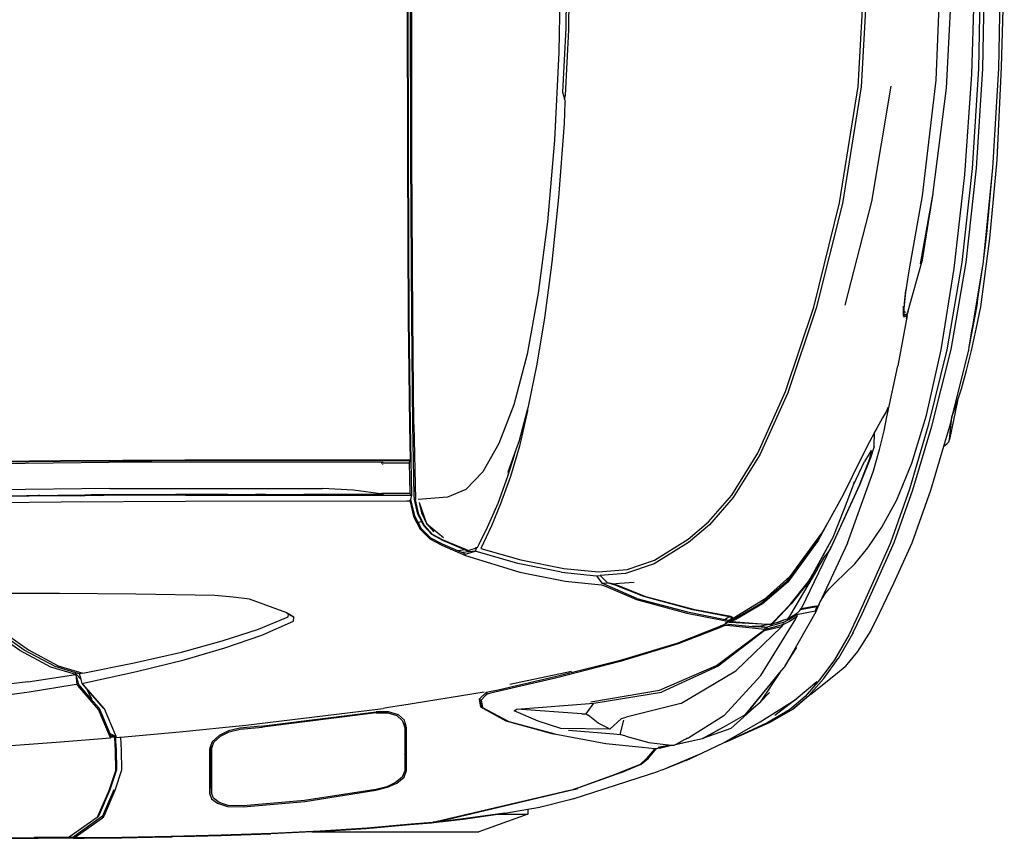
# Model space of a CAD drawing. Units: inches. Extents: x 22042254 to 25404563, y 17568978 to 17626777.
# Tile 16 of 45: x 22042342.6037 to 22042343.228, y 17568977.6632 to 17568978.1821. Entities that reach past the tile are written whole.
import ezdxf

# ---------------------------------------------------------------- set-up
doc = ezdxf.new("R2010")
doc.units = ezdxf.units.IN
doc.header["$MEASUREMENT"] = 0
doc.layers.add('A-SITE-VEHI', color=8, linetype='Continuous', lineweight=18)
doc.layers.add('Edges', color=250, linetype='Continuous')

# ---------------------------------------------------------------- blocks, each defined once
blk = doc.blocks.new('Nissan Qashqai pl')
at = {"layer": 'Edges'}
for p, q in [((10.6151, 12.8159), (10.6644, 12.8162)), ((10.6176, 12.8164), (10.6651, 12.8167)), ((10.6644, 12.8162), (10.7078, 12.8159)), ((10.6651, 12.8167), (10.666, 12.8167)), ((10.666, 12.8167), (10.677, 12.8167)), ((10.6729, 12.8157), (10.7082, 12.8156)), ((10.6809, 12.8167), (10.677, 12.8167)), ((10.7128, 12.8166), (10.6809, 12.8167)), ((10.7078, 12.8159), (10.7083, 12.8156)), ((10.7082, 12.8156), (10.7078, 12.8159)), ((10.7085, 12.8153), (10.7082, 12.8156)), ((10.7082, 12.8156), (10.7083, 12.8156)), ((10.7083, 12.8156), (10.7087, 12.8153)), ((10.7083, 12.8156), (10.7125, 12.8156)), ((10.7087, 12.8153), (10.7363, 12.7959)), ((10.7139, 12.8164), (10.7125, 12.8156)), ((10.7137, 12.8148), (10.7125, 12.8156)), ((10.7128, 12.8166), (10.7625, 12.8161)), ((10.7128, 12.8166), (10.724, 12.8166)), ((10.7139, 12.8164), (10.7148, 12.8157)), ((10.7628, 12.8158), (10.7139, 12.8164)), ((10.7148, 12.8157), (10.7429, 12.7956)), ((10.7685, 12.8161), (10.724, 12.8166)), ((10.7625, 12.8161), (10.7628, 12.8161)), ((10.7628, 12.8161), (10.8099, 12.8152)), ((10.8131, 12.8149), (10.7628, 12.8158)), ((10.7688, 12.8161), (10.7685, 12.8161)), ((10.8099, 12.8152), (10.7688, 12.8161)), ((10.8099, 12.8152), (10.8131, 12.8152)), ((10.8134, 12.8152), (10.8131, 12.8152)), ((10.8134, 12.8152), (10.8142, 12.8152)), ((10.8142, 12.8152), (10.8142, 12.8152)), ((10.8237, 12.8149), (10.8142, 12.8152)), ((10.7137, 12.8148), (10.7138, 12.8147)), ((10.7418, 12.7947), (10.7138, 12.8147)), ((10.8644, 12.8135), (10.8131, 12.8149)), ((10.8237, 12.8149), (10.864, 12.8138)), ((10.8596, 12.8138), (10.8589, 12.8138)), ((10.8642, 12.8136), (10.8596, 12.8138)), ((10.864, 12.8138), (10.8642, 12.8138)), ((10.8642, 12.8138), (10.9152, 12.812)), ((10.9158, 12.8118), (10.8644, 12.8135)), ((10.9577, 12.8101), (10.9152, 12.812)), ((10.9657, 12.8095), (10.9158, 12.8118)), ((10.9577, 12.8101), (10.9649, 12.8097)), ((10.9577, 12.8101), (11.1283, 12.8101)), ((10.9649, 12.8097), (11.0127, 12.8067)), ((11.0138, 12.8064), (10.9657, 12.8095)), ((11.0127, 12.8067), (11.0576, 12.8026)), ((11.059, 12.8023), (11.0138, 12.8064)), ((11.1783, 12.7921), (11.1283, 12.8101)), ((10.7363, 12.7959), (10.7376, 12.795)), ((10.7387, 12.794), (10.7376, 12.795)), ((10.7376, 12.795), (10.7378, 12.7946)), ((10.7432, 12.7954), (10.7426, 12.7954)), ((10.7429, 12.7956), (10.7432, 12.7954)), ((10.7441, 12.7954), (10.7432, 12.7954)), ((10.7432, 12.7954), (10.744, 12.7948)), ((11.0576, 12.8026), (11.0798, 12.8008)), ((11.0768, 12.8008), (11.059, 12.8023)), ((11.0811, 12.8004), (11.0768, 12.8008)), ((11.0798, 12.8008), (11.0872, 12.7999)), ((11.0827, 12.8001), (11.0811, 12.8004)), ((11.0827, 12.8001), (11.0813, 12.7998)), ((11.0836, 12.8002), (11.0827, 12.8001)), ((11.0856, 12.7994), (11.0827, 12.8001)), ((11.0872, 12.7999), (11.0836, 12.8002)), ((11.0836, 12.8002), (11.0882, 12.7992)), ((11.2196, 12.7681), (11.0856, 12.7994)), ((11.0883, 12.7998), (11.0872, 12.7999)), ((11.0882, 12.7992), (11.2222, 12.7676)), ((11.0883, 12.7998), (11.1123, 12.797)), ((11.1147, 12.7965), (11.0883, 12.7998)), ((11.1123, 12.797), (11.1475, 12.7921)), ((11.1547, 12.791), (11.1147, 12.7965)), ((10.7378, 12.7946), (10.7379, 12.7945)), ((10.7378, 12.7946), (10.7385, 12.7932)), ((10.7385, 12.7932), (10.7497, 12.7679)), ((10.7387, 12.794), (10.7396, 12.7922)), ((10.7396, 12.7922), (10.7507, 12.7669)), ((10.743, 12.7939), (10.7418, 12.7947)), ((10.7434, 12.793), (10.743, 12.7939)), ((10.7437, 12.7921), (10.7434, 12.793)), ((10.7438, 12.7921), (10.7437, 12.7921)), ((10.7438, 12.7921), (10.7549, 12.7666)), ((10.744, 12.7948), (10.7448, 12.793)), ((10.7448, 12.793), (10.7559, 12.7674)), ((11.1475, 12.7921), (11.1525, 12.7914)), ((11.1475, 12.7921), (11.1783, 12.7921)), ((11.1525, 12.7914), (11.1547, 12.791)), ((11.1547, 12.791), (11.1783, 12.787)), ((11.1783, 12.787), (11.1783, 12.7921)), ((11.1783, 12.787), (11.1906, 12.7849)), ((11.1906, 12.7849), (11.1909, 12.7849)), ((11.193, 12.7845), (11.1909, 12.7849)), ((10.8523, 12.7704), (10.8546, 12.7762)), ((10.8565, 12.7757), (10.8543, 12.7702)), ((10.8546, 12.7762), (10.8607, 12.7808)), ((10.8622, 12.7801), (10.8565, 12.7757)), ((10.8607, 12.7808), (10.8708, 12.7841)), ((10.8716, 12.7832), (10.8622, 12.7801)), ((10.8708, 12.7841), (10.8869, 12.7844)), ((10.887, 12.7835), (10.8716, 12.7832)), ((10.8869, 12.7844), (10.9499, 12.7789)), ((10.9498, 12.7781), (10.887, 12.7835)), ((11.0226, 12.7668), (10.9498, 12.7781)), ((10.9499, 12.7789), (11.0229, 12.7676)), ((11.2215, 12.7775), (11.193, 12.7845)), ((11.2247, 12.7764), (11.2215, 12.7775)), ((11.2247, 12.7764), (11.3124, 12.7479)), ((10.7497, 12.7679), (10.7565, 12.7473)), ((10.7507, 12.7669), (10.7575, 12.7462)), ((10.7559, 12.7674), (10.7626, 12.7467)), ((10.8523, 12.7255), (10.8523, 12.7704)), ((10.8543, 12.7702), (10.8538, 12.753)), ((10.8543, 12.7255), (10.8543, 12.7702)), ((11.0339, 12.7639), (11.0226, 12.7668)), ((11.0229, 12.7676), (11.0348, 12.7645)), ((11.2247, 12.767), (11.2163, 12.7689)), ((11.22, 12.768), (11.2196, 12.7681)), ((11.2247, 12.767), (11.22, 12.768)), ((11.2222, 12.7676), (11.2271, 12.7664)), ((11.2253, 12.7668), (11.2247, 12.767)), ((11.2304, 12.7649), (11.2253, 12.7668)), ((11.2253, 12.7668), (11.2271, 12.7664)), ((11.2271, 12.7664), (11.2296, 12.7658)), ((11.2271, 12.7664), (11.2277, 12.7662)), ((11.2277, 12.7662), (11.2296, 12.7658)), ((11.2732, 12.7496), (11.2277, 12.7662)), ((11.2704, 12.7504), (11.2304, 12.7649)), ((11.0429, 12.7597), (11.0339, 12.7639)), ((11.0348, 12.7645), (11.0444, 12.7601)), ((11.0497, 12.7542), (11.0429, 12.7597)), ((11.0444, 12.7601), (11.0516, 12.7542)), ((10.7565, 12.7473), (10.7563, 12.7273)), ((10.7575, 12.7462), (10.7572, 12.7263)), ((10.7626, 12.7467), (10.7623, 12.7269)), ((10.8528, 12.7503), (10.8535, 12.7521)), ((10.8528, 12.742), (10.8528, 12.7503)), ((10.8535, 12.7521), (10.8538, 12.753)), ((10.8538, 12.7521), (10.8535, 12.7521)), ((10.8538, 12.753), (10.8538, 12.7521)), ((10.8538, 12.7521), (10.8538, 12.7502)), ((10.8538, 12.7502), (10.8538, 12.742)), ((11.0523, 12.7475), (11.0497, 12.7542)), ((11.0516, 12.7542), (11.0543, 12.7473)), ((11.0528, 12.73), (11.0523, 12.7475)), ((11.0523, 12.7312), (11.0523, 12.7475)), ((11.0543, 12.7473), (11.0543, 12.7035)), ((11.2702, 12.7507), (11.2704, 12.7504)), ((11.2704, 12.7506), (11.2707, 12.7503)), ((11.2707, 12.7503), (11.2704, 12.7504)), ((11.2719, 12.7498), (11.2707, 12.7503)), ((11.2934, 12.741), (11.2719, 12.7498)), ((11.2732, 12.7496), (11.2946, 12.7409)), ((11.3161, 12.7467), (11.3124, 12.7479)), ((11.3161, 12.7467), (11.3376, 12.7381)), ((11.3192, 12.7454), (11.3566, 12.7294)), ((10.8528, 12.742), (10.8538, 12.742)), ((10.8528, 12.7419), (10.8528, 12.742)), ((10.8538, 12.7419), (10.8528, 12.7419)), ((10.8528, 12.7242), (10.8528, 12.7419)), ((10.8538, 12.742), (10.8538, 12.7419)), ((10.8538, 12.7214), (10.8538, 12.7419)), ((11.3, 12.735), (11.2934, 12.741)), ((11.2946, 12.7409), (11.3018, 12.7346)), ((11.3081, 12.7253), (11.3, 12.735)), ((11.3018, 12.7346), (11.3103, 12.7249)), ((11.3405, 12.7369), (11.3376, 12.7381)), ((11.3405, 12.7369), (11.3566, 12.7294)), ((10.7563, 12.7273), (10.7553, 12.7134)), ((10.7572, 12.7263), (10.7563, 12.7126)), ((10.7623, 12.7269), (10.7615, 12.7131)), ((10.8528, 12.7242), (10.8523, 12.7255)), ((10.8543, 12.7255), (10.8569, 12.7184)), ((11.0523, 12.7312), (11.0528, 12.73)), ((11.0523, 12.7287), (11.0523, 12.7312)), ((11.0528, 12.7274), (11.0523, 12.7287)), ((11.0523, 12.7037), (11.0523, 12.7287)), ((11.0528, 12.7274), (11.0528, 12.73)), ((11.0528, 12.73), (11.0538, 12.7273)), ((11.0528, 12.7274), (11.0528, 12.6985)), ((11.0538, 12.7273), (11.0538, 12.7018)), ((11.2956, 12.7234), (11.3085, 12.7247)), ((11.3086, 12.7247), (11.3081, 12.7253)), ((11.3081, 12.7253), (11.3087, 12.7247)), ((11.3085, 12.7247), (11.3086, 12.7247)), ((11.3086, 12.7247), (11.3087, 12.7247)), ((11.3087, 12.7247), (11.3103, 12.7249)), ((11.3103, 12.7249), (11.3103, 12.7249)), ((11.3103, 12.7249), (11.3106, 12.7249)), ((11.3106, 12.7249), (11.314, 12.7238)), ((11.3566, 12.7294), (11.3796, 12.7187)), ((10.6318, 12.7228), (10.6955, 12.7184)), ((10.6955, 12.7184), (10.7509, 12.714)), ((10.8538, 12.7214), (10.8528, 12.7242)), ((10.855, 12.7181), (10.8538, 12.7214)), ((10.8622, 12.7114), (10.855, 12.7181)), ((10.8569, 12.7184), (10.8637, 12.712)), ((11.2091, 12.7103), (11.2583, 12.7196)), ((11.2583, 12.7196), (11.2956, 12.7234)), ((11.2787, 12.7123), (11.3022, 12.7186)), ((11.3022, 12.7186), (11.3252, 12.7213)), ((11.317, 12.7227), (11.3119, 12.7236)), ((11.3132, 12.7243), (11.3256, 12.7215)), ((11.314, 12.7238), (11.317, 12.7227)), ((11.314, 12.7238), (11.3242, 12.7216)), ((11.3242, 12.7216), (11.317, 12.7227)), ((11.3198, 12.7211), (11.3252, 12.7213)), ((11.3242, 12.7216), (11.3256, 12.7215)), ((11.3252, 12.7213), (11.3283, 12.7214)), ((11.3256, 12.7215), (11.3283, 12.7214)), ((11.3283, 12.7214), (11.3297, 12.7206)), ((11.3297, 12.7206), (11.3446, 12.7173)), ((11.3297, 12.7206), (11.3302, 12.7203)), ((11.3302, 12.7203), (11.3446, 12.7173)), ((11.3302, 12.7203), (11.3394, 12.7152)), ((11.3394, 12.7152), (11.3434, 12.7138)), ((11.3394, 12.7152), (11.342, 12.7137)), ((11.3446, 12.7173), (11.3571, 12.7146)), ((11.3583, 12.7142), (11.3571, 12.7146)), ((11.3571, 12.7146), (11.3821, 12.7008)), ((11.3796, 12.7187), (11.4164, 12.6974)), ((11.3796, 12.7187), (11.3807, 12.7182)), ((11.3807, 12.7182), (11.4267, 12.6979)), ((11.4228, 12.6989), (11.3807, 12.7182)), ((10.7501, 12.7114), (10.7387, 12.6849)), ((10.7507, 12.7098), (10.7397, 12.684)), ((10.7563, 12.7109), (10.7449, 12.6843)), ((10.7507, 12.7132), (10.7501, 12.7114)), ((10.7506, 12.7111), (10.7507, 12.7132)), ((10.7507, 12.7132), (10.7509, 12.714)), ((10.751, 12.7132), (10.7507, 12.7132)), ((10.7511, 12.7107), (10.7507, 12.7098)), ((10.7524, 12.7106), (10.7507, 12.7098)), ((10.7522, 12.7131), (10.7509, 12.714)), ((10.7516, 12.7131), (10.7509, 12.714)), ((10.7519, 12.7128), (10.7511, 12.7107)), ((10.7522, 12.7131), (10.7516, 12.7131)), ((10.7519, 12.7128), (10.7516, 12.7131)), ((10.7526, 12.7124), (10.7519, 12.7128)), ((10.7553, 12.7134), (10.7522, 12.7131)), ((10.7524, 12.7106), (10.7526, 12.7124)), ((10.7556, 12.7122), (10.7524, 12.7106)), ((10.7526, 12.7124), (10.7526, 12.7127)), ((10.7532, 12.712), (10.7526, 12.7124)), ((10.7556, 12.7122), (10.7532, 12.712)), ((10.7561, 12.7125), (10.7556, 12.7122)), ((10.7561, 12.7125), (10.7563, 12.7126)), ((10.7563, 12.7125), (10.7561, 12.7125)), ((10.7563, 12.7123), (10.7561, 12.7123)), ((10.7563, 12.7126), (10.7573, 12.7135)), ((10.7563, 12.7126), (10.7563, 12.7125)), ((10.7569, 12.7125), (10.7563, 12.7109)), ((10.7569, 12.7125), (10.7563, 12.7125)), ((10.7563, 12.7125), (10.7563, 12.7123)), ((10.7573, 12.7135), (10.7569, 12.7125)), ((10.7573, 12.7135), (10.7604, 12.7132)), ((10.7604, 12.7132), (10.7615, 12.7131)), ((10.7615, 12.7131), (10.8218, 12.7077)), ((10.8218, 12.7077), (10.8896, 12.7008)), ((10.8718, 12.7068), (10.8622, 12.7114)), ((10.8637, 12.712), (10.8727, 12.7077)), ((10.8836, 12.7041), (10.8718, 12.7068)), ((10.8727, 12.7077), (10.8839, 12.7051)), ((10.8839, 12.7051), (10.9067, 12.7029)), ((11.156, 12.6966), (11.203, 12.7093)), ((11.1589, 12.6971), (11.2062, 12.7098)), ((11.2121, 12.7043), (11.189, 12.6968)), ((11.203, 12.7093), (11.2091, 12.7103)), ((11.2062, 12.7098), (11.2091, 12.7103)), ((11.2622, 12.7051), (11.2121, 12.7043)), ((11.2199, 12.706), (11.2666, 12.7097)), ((11.2622, 12.7051), (11.2601, 12.7037)), ((11.2743, 12.6942), (11.2622, 12.7051)), ((11.2666, 12.7097), (11.2729, 12.7104)), ((11.2787, 12.7123), (11.2729, 12.7104)), ((11.2729, 12.7104), (11.2766, 12.6957)), ((11.379, 12.6915), (11.3434, 12.7138)), ((11.3583, 12.7142), (11.3821, 12.7008)), ((11.3864, 12.7044), (11.3583, 12.7142)), ((11.4163, 12.6775), (11.3864, 12.7044)), ((10.9054, 12.702), (10.8836, 12.7041)), ((10.8896, 12.7008), (11.0304, 12.6838)), ((10.9054, 12.702), (11.0232, 12.6871)), ((11.0231, 12.6882), (10.9067, 12.7029)), ((11.0443, 12.6911), (11.0501, 12.6964)), ((11.052, 12.6958), (11.0458, 12.6903)), ((11.0501, 12.6964), (11.0523, 12.7037)), ((11.0528, 12.6985), (11.052, 12.6958)), ((11.0538, 12.7018), (11.0528, 12.6985)), ((11.0543, 12.7035), (11.0538, 12.7018)), ((11.1298, 12.6823), (11.156, 12.6966)), ((11.1365, 12.6851), (11.1589, 12.6971)), ((11.189, 12.6968), (11.1644, 12.6862)), ((11.2505, 12.6987), (11.2401, 12.6908)), ((11.2601, 12.7037), (11.2505, 12.6987)), ((11.2743, 12.6942), (11.2791, 12.6927)), ((11.3821, 12.7008), (11.4014, 12.69)), ((11.4164, 12.6974), (11.4531, 12.6744)), ((11.4243, 12.6982), (11.4228, 12.6989)), ((11.4464, 12.6853), (11.4243, 12.6982)), ((11.4267, 12.6979), (11.4498, 12.6844)), ((10.7387, 12.6849), (10.7177, 12.6604)), ((10.7449, 12.6843), (10.7232, 12.6594)), ((11.0231, 12.6882), (11.035, 12.6883)), ((11.0358, 12.6872), (11.0232, 12.6871)), ((11.035, 12.6883), (11.0443, 12.6911)), ((11.0458, 12.6903), (11.0358, 12.6872)), ((11.1319, 12.6827), (11.1365, 12.6851)), ((11.1644, 12.6862), (11.1672, 12.6844)), ((11.2337, 12.6892), (11.1672, 12.6844)), ((11.1672, 12.6844), (11.2459, 12.6785)), ((11.2337, 12.6892), (11.2382, 12.6892)), ((11.2382, 12.6892), (11.2401, 12.6908)), ((11.2382, 12.6892), (11.2459, 12.6785)), ((11.335, 12.6786), (11.2791, 12.6927)), ((11.379, 12.6915), (11.417, 12.6499)), ((11.4014, 12.69), (11.4022, 12.6894)), ((11.4014, 12.69), (11.4265, 12.6594)), ((11.4022, 12.6894), (11.4163, 12.6775)), ((11.4022, 12.6894), (11.4265, 12.6594)), ((11.4531, 12.6744), (11.4314, 12.6911)), ((11.4624, 12.6717), (11.4464, 12.6853)), ((11.4498, 12.6844), (11.4662, 12.6706)), ((11.4681, 12.6691), (11.4498, 12.6844)), ((10.6678, 12.6672), (10.6152, 12.674)), ((10.7334, 12.6766), (10.7186, 12.6593)), ((10.7438, 12.6836), (10.7265, 12.6635)), ((10.7265, 12.6635), (10.7316, 12.6741)), ((10.7397, 12.684), (10.7334, 12.6766)), ((11.0357, 12.6829), (11.0304, 12.6838)), ((11.0491, 12.6807), (11.0357, 12.6829)), ((11.0449, 12.6812), (11.0448, 12.6812)), ((11.0492, 12.6807), (11.0491, 12.6807)), ((11.1336, 12.667), (11.0492, 12.6807)), ((11.1285, 12.6745), (11.1298, 12.6823)), ((11.1293, 12.6736), (11.1285, 12.6745)), ((11.1306, 12.6812), (11.1293, 12.6736)), ((11.1306, 12.6752), (11.1319, 12.6827)), ((11.1319, 12.6827), (11.1306, 12.6812)), ((11.1347, 12.671), (11.1306, 12.6752)), ((11.2428, 12.6769), (11.3132, 12.6652)), ((11.2459, 12.6785), (11.3153, 12.6672)), ((11.335, 12.6786), (11.3915, 12.6453)), ((11.4366, 12.6471), (11.4163, 12.6775)), ((11.4163, 12.6775), (11.4259, 12.6674)), ((11.4742, 12.6567), (11.4531, 12.6744)), ((10.7137, 12.6595), (10.6678, 12.6672)), ((11.1353, 12.6677), (11.1293, 12.6736)), ((11.1366, 12.6691), (11.1347, 12.671)), ((11.1358, 12.6676), (11.1353, 12.6677)), ((11.1358, 12.6676), (11.1366, 12.6691)), ((11.148, 12.665), (11.1358, 12.6676)), ((11.1401, 12.6682), (11.1366, 12.6691)), ((11.2066, 12.6527), (11.1401, 12.6682)), ((11.2063, 12.6515), (11.148, 12.665)), ((11.3132, 12.6652), (11.3715, 12.6398)), ((11.3733, 12.6404), (11.3153, 12.6672)), ((11.4774, 12.6543), (11.4624, 12.6717)), ((11.4662, 12.6706), (11.4815, 12.6531)), ((11.4681, 12.6691), (11.4936, 12.6491)), ((10.6664, 12.6566), (10.6144, 12.6629)), ((10.6664, 12.6566), (10.7155, 12.649)), ((10.7165, 12.6591), (10.7137, 12.6595)), ((10.7186, 12.6593), (10.7155, 12.649)), ((10.7155, 12.649), (10.7165, 12.6591)), ((10.7209, 12.654), (10.7155, 12.6485)), ((10.7177, 12.6604), (10.7165, 12.6591)), ((10.7209, 12.654), (10.7192, 12.6484)), ((10.7221, 12.6581), (10.7209, 12.654)), ((10.7232, 12.6594), (10.7221, 12.6581)), ((10.7221, 12.6581), (10.7224, 12.6587)), ((10.7221, 12.6581), (10.7247, 12.6575)), ((10.7265, 12.6635), (10.7224, 12.6587)), ((10.7247, 12.6575), (10.7776, 12.646)), ((11.2232, 12.6458), (11.1598, 12.6594)), ((11.4265, 12.6594), (11.4366, 12.6471)), ((11.4924, 12.6339), (11.4774, 12.6543)), ((10.7155, 12.649), (10.69, 12.6414)), ((10.7155, 12.6473), (10.6943, 12.641)), ((10.6976, 12.6401), (10.7228, 12.6477)), ((10.7155, 12.649), (10.7155, 12.6485)), ((10.7155, 12.6485), (10.7155, 12.6473)), ((10.7192, 12.6484), (10.7155, 12.6473)), ((10.7228, 12.6477), (10.7192, 12.6484)), ((10.7228, 12.6477), (10.7754, 12.637)), ((10.7776, 12.646), (10.8264, 12.6341)), ((11.272, 12.6349), (11.2063, 12.6515)), ((11.2728, 12.6357), (11.2066, 12.6527)), ((11.3915, 12.6453), (11.4381, 12.6002)), ((11.417, 12.6499), (11.4529, 12.5922)), ((11.4366, 12.6471), (11.4408, 12.6419)), ((11.4815, 12.6531), (11.4963, 12.6328)), ((11.4936, 12.6491), (11.5033, 12.6408)), ((10.69, 12.6414), (10.6583, 12.6245)), ((10.6943, 12.641), (10.6627, 12.6241)), ((10.6671, 12.6238), (10.6976, 12.6401)), ((10.7754, 12.637), (10.8239, 12.6261)), ((10.8264, 12.6341), (10.8682, 12.6216)), ((11.3311, 12.6172), (11.272, 12.6349)), ((11.3323, 12.6178), (11.2728, 12.6357)), ((11.3715, 12.6398), (11.4177, 12.6052)), ((11.4203, 12.6044), (11.3733, 12.6404)), ((11.4408, 12.6419), (11.4411, 12.6414)), ((11.4411, 12.6414), (11.4411, 12.6414)), ((11.4414, 12.6409), (11.4411, 12.6414)), ((11.4414, 12.6409), (11.447, 12.6315)), ((11.4455, 12.6336), (11.4414, 12.6409)), ((11.5074, 12.608), (11.4924, 12.6339)), ((11.5158, 12.6256), (11.5033, 12.6408)), ((10.6583, 12.6245), (10.6215, 12.5986)), ((10.6627, 12.6241), (10.6261, 12.5984)), ((10.6306, 12.5982), (10.6671, 12.6238)), ((10.8239, 12.6261), (10.8653, 12.6144)), ((11.447, 12.6315), (11.4455, 12.6336)), ((11.4455, 12.6336), (11.4462, 12.6324)), ((11.447, 12.6315), (11.4462, 12.6324)), ((11.4732, 12.585), (11.4462, 12.6324)), ((11.447, 12.6315), (11.447, 12.6314)), ((11.4536, 12.6215), (11.447, 12.6314)), ((11.4964, 12.6326), (11.4963, 12.6328)), ((11.4964, 12.6326), (11.5113, 12.6069)), ((11.5295, 12.6041), (11.5158, 12.6256)), ((10.8653, 12.6144), (10.9026, 12.6025)), ((10.8682, 12.6216), (10.9059, 12.6087)), ((11.3751, 12.5999), (11.3311, 12.6172)), ((11.3747, 12.6011), (11.3323, 12.6178)), ((10.9059, 12.6087), (10.9384, 12.5945)), ((11.4177, 12.6052), (11.4193, 12.6042)), ((11.4192, 12.6045), (11.4194, 12.6042)), ((11.4194, 12.6042), (11.4193, 12.6042)), ((11.4193, 12.6042), (11.4196, 12.604)), ((11.4194, 12.6042), (11.4196, 12.604)), ((11.4196, 12.6042), (11.4194, 12.6042)), ((11.4196, 12.604), (11.4201, 12.6036)), ((11.4198, 12.6041), (11.4201, 12.6036)), ((11.4201, 12.6036), (11.4212, 12.603)), ((11.4292, 12.6024), (11.4203, 12.6044)), ((11.4229, 12.6025), (11.4203, 12.6044)), ((11.5165, 12.5882), (11.5074, 12.608)), ((11.5113, 12.6068), (11.5113, 12.6069)), ((11.5113, 12.6068), (11.5206, 12.5869)), ((11.5384, 12.5859), (11.5295, 12.6041)), ((10.9026, 12.6025), (10.933, 12.5901)), ((10.9384, 12.5945), (10.9386, 12.5905)), ((11.3411, 12.5863), (11.3795, 12.5939)), ((11.38, 12.5988), (11.3747, 12.6011)), ((11.3751, 12.5999), (11.3762, 12.5999)), ((11.3752, 12.5998), (11.3751, 12.5999)), ((11.3763, 12.5998), (11.3752, 12.5998)), ((11.3764, 12.5993), (11.3752, 12.5998)), ((11.3792, 12.5982), (11.3764, 12.5993)), ((11.3792, 12.5982), (11.3793, 12.5979)), ((11.3792, 12.5982), (11.3804, 12.5972)), ((11.3795, 12.5939), (11.3834, 12.5947)), ((11.3853, 12.5993), (11.38, 12.5988)), ((11.3804, 12.5972), (11.4082, 12.5998)), ((11.3827, 12.5953), (11.3804, 12.5972)), ((11.3804, 12.5926), (11.3841, 12.5933)), ((11.3811, 12.5958), (11.3808, 12.5961)), ((11.3834, 12.5947), (11.3827, 12.5953)), ((11.3846, 12.5953), (11.3829, 12.5952)), ((11.3829, 12.5952), (11.3849, 12.5951)), ((11.388, 12.591), (11.3829, 12.5952)), ((11.3834, 12.5947), (11.3841, 12.5933)), ((11.3846, 12.5953), (11.4248, 12.5976)), ((11.3846, 12.5953), (11.3846, 12.5953)), ((11.3851, 12.5951), (11.3846, 12.5953)), ((11.3846, 12.5953), (11.3849, 12.5951)), ((11.3849, 12.5951), (11.3851, 12.5951)), ((11.3882, 12.5923), (11.3849, 12.5951)), ((11.3851, 12.5951), (11.3867, 12.5949)), ((11.4171, 12.5766), (11.3851, 12.5951)), ((11.4212, 12.603), (11.3853, 12.5993)), ((11.3867, 12.5949), (11.3915, 12.5951)), ((11.3914, 12.5926), (11.3867, 12.5949)), ((11.3915, 12.5951), (11.4266, 12.5977)), ((11.409, 12.5999), (11.4082, 12.5998)), ((11.4164, 12.5998), (11.4082, 12.5998)), ((11.4152, 12.6004), (11.409, 12.5999)), ((11.409, 12.5999), (11.4163, 12.5999)), ((11.4173, 12.6006), (11.4152, 12.6004)), ((11.4163, 12.5999), (11.4152, 12.6004)), ((11.4163, 12.5999), (11.4186, 12.5999)), ((11.4164, 12.5998), (11.4163, 12.5999)), ((11.4181, 12.5998), (11.4164, 12.5998)), ((11.4169, 12.5996), (11.4164, 12.5998)), ((11.4252, 12.598), (11.4169, 12.5996)), ((11.4176, 12.6007), (11.4173, 12.6006)), ((11.418, 12.6006), (11.4173, 12.6006)), ((11.4215, 12.601), (11.4176, 12.6007)), ((11.418, 12.6006), (11.4176, 12.6007)), ((11.4204, 12.6002), (11.418, 12.6006)), ((11.4194, 12.6), (11.418, 12.6006)), ((11.4212, 12.603), (11.4215, 12.601)), ((11.4218, 12.6028), (11.4212, 12.603)), ((11.4215, 12.601), (11.4219, 12.6009)), ((11.4222, 12.6029), (11.4218, 12.6028)), ((11.4229, 12.6025), (11.4218, 12.6028)), ((11.4219, 12.6009), (11.4222, 12.6005)), ((11.4219, 12.6009), (11.4224, 12.6008)), ((11.4224, 12.6008), (11.4226, 12.6006)), ((11.4224, 12.6008), (11.423, 12.6006)), ((11.4315, 12.6002), (11.4229, 12.6025)), ((11.423, 12.6006), (11.4229, 12.6025)), ((11.44, 12.5959), (11.423, 12.6006)), ((11.4248, 12.5976), (11.4266, 12.5977)), ((11.4266, 12.5977), (11.4252, 12.598)), ((11.4266, 12.5977), (11.4268, 12.5977)), ((11.4268, 12.5977), (11.4296, 12.5954)), ((11.4268, 12.5977), (11.4278, 12.5977)), ((11.4303, 12.5956), (11.4278, 12.5977)), ((11.4278, 12.5977), (11.43, 12.5969)), ((11.4381, 12.6002), (11.4292, 12.6024)), ((11.4296, 12.5954), (11.4469, 12.5773)), ((11.4337, 12.5962), (11.43, 12.5969)), ((11.43, 12.5969), (11.4361, 12.5948)), ((11.4479, 12.5766), (11.4303, 12.5956)), ((11.4403, 12.5978), (11.4315, 12.6002)), ((11.4397, 12.5937), (11.4337, 12.5962)), ((11.4361, 12.5948), (11.4406, 12.5932)), ((11.4381, 12.6002), (11.4403, 12.5978)), ((11.4406, 12.5932), (11.4397, 12.5937)), ((11.4403, 12.5978), (11.44, 12.5959)), ((11.44, 12.5959), (11.4457, 12.5928)), ((11.4462, 12.5947), (11.4403, 12.5978)), ((11.452, 12.591), (11.4462, 12.5947)), ((10.9316, 12.586), (10.8932, 12.572)), ((10.9316, 12.586), (10.9334, 12.5872)), ((10.932, 12.5862), (10.9316, 12.586)), ((10.9335, 12.5871), (10.932, 12.5862)), ((10.933, 12.5901), (10.9334, 12.5872)), ((10.9334, 12.5872), (10.9386, 12.5905)), ((10.9334, 12.5872), (10.9335, 12.5871)), ((10.9386, 12.5905), (10.9335, 12.5871)), ((11.2895, 12.5724), (11.3411, 12.5863)), ((11.29, 12.5711), (11.3419, 12.585)), ((11.3419, 12.585), (11.3804, 12.5926)), ((11.3847, 12.5899), (11.3474, 12.5827)), ((11.3863, 12.5898), (11.3493, 12.5828)), ((11.3847, 12.5899), (11.3804, 12.5926)), ((11.3847, 12.5899), (11.3848, 12.5899)), ((11.388, 12.591), (11.3848, 12.5899)), ((11.3895, 12.5912), (11.3863, 12.5898)), ((11.3886, 12.5919), (11.3872, 12.5927)), ((11.3882, 12.5923), (11.3886, 12.5919)), ((11.3886, 12.5919), (11.3895, 12.5912)), ((11.3892, 12.5916), (11.3886, 12.5919)), ((11.3923, 12.5894), (11.3895, 12.5912)), ((11.4187, 12.5768), (11.3914, 12.5926)), ((11.4203, 12.5724), (11.3923, 12.5894)), ((11.4406, 12.5932), (11.4442, 12.592)), ((11.4442, 12.592), (11.4497, 12.589)), ((11.4462, 12.5893), (11.4442, 12.592)), ((11.4457, 12.5928), (11.4512, 12.5893)), ((11.475, 12.5409), (11.4462, 12.5893)), ((11.4497, 12.589), (11.4498, 12.5889)), ((11.4535, 12.5876), (11.4498, 12.5889)), ((11.4498, 12.5889), (11.4549, 12.5855)), ((11.4512, 12.5893), (11.4535, 12.5876)), ((11.4539, 12.5897), (11.452, 12.591)), ((11.4529, 12.5922), (11.4542, 12.5894)), ((11.4535, 12.5876), (11.4532, 12.5882)), ((11.4535, 12.5876), (11.4542, 12.5894)), ((11.4535, 12.5876), (11.4728, 12.5838)), ((11.4542, 12.5894), (11.4539, 12.5897)), ((11.4549, 12.5855), (11.4568, 12.5836)), ((11.4564, 12.5833), (11.4567, 12.5833)), ((11.4568, 12.5836), (11.4571, 12.5833)), ((11.4571, 12.5833), (11.4573, 12.583)), ((11.4732, 12.585), (11.4728, 12.5838)), ((11.4728, 12.5838), (11.4742, 12.5797)), ((11.4728, 12.5838), (11.4746, 12.5796)), ((11.4758, 12.5791), (11.4732, 12.585)), ((11.5306, 12.5573), (11.5165, 12.5882)), ((11.5206, 12.5869), (11.5349, 12.5559)), ((11.5527, 12.5559), (11.5384, 12.5859)), ((11.3474, 12.5827), (11.2972, 12.5692)), ((11.3493, 12.5828), (11.2993, 12.5695)), ((11.3474, 12.5827), (11.3474, 12.5827)), ((11.4433, 12.5543), (11.4171, 12.5766)), ((11.4447, 12.5545), (11.4187, 12.5768)), ((11.4469, 12.5773), (11.4659, 12.5539)), ((11.4654, 12.5548), (11.4479, 12.5766)), ((11.4569, 12.583), (11.4565, 12.5831)), ((11.4573, 12.583), (11.4578, 12.5822)), ((11.4704, 12.5803), (11.4573, 12.583)), ((11.4573, 12.5823), (11.4574, 12.5822)), ((11.4573, 12.5823), (11.4573, 12.5823)), ((11.4576, 12.5822), (11.4574, 12.5822)), ((11.4578, 12.5822), (11.4588, 12.5807)), ((11.4605, 12.5816), (11.4578, 12.5822)), ((11.4588, 12.5807), (11.4895, 12.5178)), ((11.4713, 12.5794), (11.4605, 12.5816)), ((11.4742, 12.5797), (11.4704, 12.5803)), ((11.4744, 12.5792), (11.4713, 12.5794)), ((11.4742, 12.5797), (11.4744, 12.5792)), ((11.4745, 12.5797), (11.4742, 12.5797)), ((11.4745, 12.5792), (11.4744, 12.5792)), ((11.4745, 12.5792), (11.4745, 12.5797)), ((11.4745, 12.5797), (11.4746, 12.5796)), ((11.4748, 12.5792), (11.4745, 12.5792)), ((11.4746, 12.5796), (11.4748, 12.5792)), ((11.4746, 12.5796), (11.4758, 12.5791)), ((11.4758, 12.5791), (11.4748, 12.5792)), ((11.4758, 12.5791), (11.4759, 12.579)), ((11.4759, 12.579), (11.4778, 12.5746)), ((11.4759, 12.579), (11.4771, 12.576)), ((11.5057, 12.5145), (11.4771, 12.576)), ((11.4778, 12.5746), (11.4826, 12.5669)), ((10.6988, 12.5662), (10.5892, 12.5659)), ((10.7769, 12.5667), (10.6988, 12.5662)), ((10.858, 12.5683), (10.7769, 12.5667)), ((10.8766, 12.5697), (10.858, 12.5683)), ((10.8932, 12.572), (10.8766, 12.5697)), ((11.29, 12.5711), (11.2541, 12.5557)), ((11.2586, 12.5591), (11.2895, 12.5724)), ((11.2972, 12.5692), (11.2677, 12.5575)), ((11.2993, 12.5695), (11.2705, 12.5579)), ((11.4467, 12.5488), (11.4203, 12.5724)), ((11.4826, 12.5669), (11.4869, 12.5615)), ((11.1702, 12.5444), (11.2166, 12.5534)), ((11.2166, 12.5534), (11.2538, 12.5571)), ((11.2488, 12.548), (11.2541, 12.5557)), ((11.2599, 12.5552), (11.2524, 12.5477)), ((11.2538, 12.5571), (11.2586, 12.5591)), ((11.2541, 12.5557), (11.2599, 12.5552)), ((11.2677, 12.5575), (11.2599, 12.5552)), ((11.265, 12.5563), (11.2599, 12.5552)), ((11.2705, 12.5579), (11.265, 12.5563)), ((11.265, 12.5563), (11.2724, 12.5557)), ((11.2724, 12.5557), (11.2874, 12.5544)), ((11.4745, 12.5116), (11.4433, 12.5543)), ((11.4758, 12.5118), (11.4447, 12.5545)), ((11.4633, 12.5594), (11.4897, 12.5108)), ((11.4654, 12.5548), (11.4659, 12.5539)), ((11.4659, 12.5539), (11.4674, 12.5512)), ((11.4869, 12.5615), (11.4933, 12.555)), ((11.5131, 12.5356), (11.4933, 12.555)), ((11.5496, 12.5141), (11.5306, 12.5573)), ((11.5349, 12.5559), (11.5535, 12.5139)), ((11.5716, 12.5145), (11.5527, 12.5559)), ((11.1144, 12.5271), (11.1702, 12.5444)), ((11.2127, 12.5443), (11.1683, 12.5354)), ((11.2127, 12.5443), (11.2488, 12.548)), ((11.2152, 12.5404), (11.2509, 12.5439)), ((11.2488, 12.548), (11.2524, 12.5477)), ((11.2509, 12.5439), (11.28, 12.5414)), ((11.2785, 12.5455), (11.2524, 12.5477)), ((11.3076, 12.5358), (11.2785, 12.5455)), ((11.4801, 12.503), (11.4467, 12.5488)), ((11.4675, 12.551), (11.4674, 12.5512)), ((11.4675, 12.551), (11.4703, 12.546)), ((11.4703, 12.546), (11.4704, 12.5458)), ((11.4704, 12.5458), (11.4909, 12.5085)), ((11.4704, 12.5458), (11.4897, 12.5108)), ((11.1683, 12.5354), (11.1244, 12.5227)), ((11.1712, 12.5317), (11.2152, 12.5404)), ((11.28, 12.5414), (11.3082, 12.532)), ((11.3428, 12.5139), (11.3076, 12.5358)), ((11.475, 12.5409), (11.4828, 12.5276)), ((11.5131, 12.5356), (11.5265, 12.5194)), ((11.0902, 12.5166), (11.1144, 12.5271)), ((11.107, 12.5224), (11.1116, 12.5243)), ((11.1116, 12.5243), (11.1147, 12.5257)), ((11.1244, 12.5227), (11.1116, 12.5243)), ((11.1147, 12.5257), (11.1244, 12.5227)), ((11.1259, 12.5194), (11.1244, 12.5227)), ((11.1244, 12.5227), (11.126, 12.5194)), ((11.1302, 12.52), (11.1712, 12.5317)), ((11.3082, 12.532), (11.3425, 12.5106)), ((11.488, 12.5208), (11.4828, 12.5276)), ((11.0779, 12.5103), (11.0902, 12.5166)), ((11.0787, 12.5092), (11.0908, 12.5153)), ((11.0908, 12.5153), (11.107, 12.5224)), ((11.1138, 12.5213), (11.0912, 12.5117)), ((11.1149, 12.5212), (11.0917, 12.5114)), ((11.1138, 12.5213), (11.107, 12.5224)), ((11.1139, 12.5213), (11.1138, 12.5213)), ((11.1164, 12.5224), (11.1139, 12.5213)), ((11.1172, 12.5222), (11.1149, 12.5212)), ((11.1164, 12.5224), (11.1174, 12.5223)), ((11.1173, 12.5222), (11.1172, 12.5222)), ((11.1174, 12.5223), (11.1173, 12.5222)), ((11.12, 12.5215), (11.1174, 12.5223)), ((11.1246, 12.5199), (11.12, 12.5215)), ((11.1259, 12.5194), (11.1246, 12.5199)), ((11.126, 12.5193), (11.1247, 12.5197)), ((11.126, 12.5193), (11.1248, 12.5195)), ((11.1251, 12.5189), (11.126, 12.5193)), ((11.126, 12.5193), (11.1259, 12.5194)), ((11.126, 12.5194), (11.1259, 12.5194)), ((11.126, 12.5194), (11.1261, 12.5193)), ((11.1264, 12.5192), (11.126, 12.5194)), ((11.1263, 12.5186), (11.126, 12.5193)), ((11.1261, 12.5193), (11.126, 12.5193)), ((11.1261, 12.5193), (11.1263, 12.5188)), ((11.1264, 12.5192), (11.1261, 12.5193)), ((11.1277, 12.5167), (11.1264, 12.5192)), ((11.1369, 12.4986), (11.1277, 12.5167)), ((11.1412, 12.4969), (11.1302, 12.52)), ((11.3645, 12.4958), (11.3428, 12.5139)), ((11.5179, 12.4551), (11.488, 12.5208)), ((11.4898, 12.5172), (11.4895, 12.5178)), ((11.4898, 12.5172), (11.49, 12.5167)), ((11.49, 12.5167), (11.5179, 12.4551)), ((11.5057, 12.5145), (11.5325, 12.4404)), ((11.5265, 12.5194), (11.541, 12.4982)), ((11.5691, 12.4592), (11.5496, 12.5141)), ((11.5535, 12.5139), (11.5726, 12.46)), ((11.5908, 12.4606), (11.5716, 12.5145)), ((11.0682, 12.5004), (11.0779, 12.5103)), ((11.0692, 12.4996), (11.0787, 12.5092)), ((11.0802, 12.5057), (11.0718, 12.4967)), ((11.0809, 12.5056), (11.0727, 12.4966)), ((11.0747, 12.4944), (11.092, 12.5087)), ((11.0747, 12.4944), (11.0821, 12.5029)), ((11.0912, 12.5117), (11.0802, 12.5057)), ((11.0917, 12.5114), (11.0809, 12.5056)), ((11.3425, 12.5106), (11.3635, 12.4929)), ((11.4788, 12.5052), (11.4745, 12.5116)), ((11.4852, 12.494), (11.4758, 12.5118)), ((11.4801, 12.503), (11.4788, 12.5052)), ((11.4852, 12.494), (11.4801, 12.503)), ((11.4897, 12.5108), (11.4909, 12.5085)), ((11.4909, 12.5085), (11.5028, 12.4792)), ((11.0614, 12.4872), (11.0682, 12.5004)), ((11.0624, 12.4866), (11.0658, 12.4932)), ((11.0658, 12.4932), (11.0692, 12.4996)), ((11.0658, 12.4932), (11.0698, 12.4925)), ((11.0698, 12.4925), (11.0659, 12.4848)), ((11.0727, 12.4966), (11.0669, 12.4849)), ((11.0671, 12.4731), (11.0747, 12.4944)), ((11.0696, 12.4836), (11.0747, 12.4944)), ((11.0718, 12.4967), (11.0698, 12.4925)), ((11.1475, 12.4741), (11.1369, 12.4986)), ((11.1505, 12.4742), (11.1412, 12.4969)), ((11.3635, 12.4929), (11.3872, 12.4654)), ((11.3888, 12.4678), (11.3645, 12.4958)), ((11.5013, 12.4651), (11.4852, 12.494)), ((11.541, 12.4982), (11.5562, 12.4701)), ((11.0581, 12.4738), (11.0614, 12.4872)), ((11.0582, 12.47), (11.0624, 12.4866)), ((11.0659, 12.4848), (11.063, 12.4728)), ((11.0669, 12.4849), (11.0641, 12.4733)), ((11.0671, 12.4731), (11.0696, 12.4836)), ((10.5572, 12.4737), (10.7004, 12.4722)), ((11.0575, 12.4714), (11.0581, 12.4738)), ((11.063, 12.4728), (11.0622, 12.4697)), ((11.0641, 12.4733), (11.0632, 12.47)), ((11.1577, 12.4465), (11.1475, 12.4741)), ((11.1605, 12.4465), (11.1505, 12.4742)), ((11.5028, 12.4792), (11.5118, 12.4548)), ((10.7, 12.4662), (10.5566, 12.4677)), ((10.5576, 12.4675), (10.6649, 12.4659)), ((10.5866, 12.467), (10.6649, 12.4659)), ((10.6649, 12.4659), (10.6786, 12.4658)), ((10.6649, 12.4659), (10.6772, 12.4657)), ((10.6786, 12.4657), (10.6772, 12.4657)), ((10.6786, 12.4658), (10.6786, 12.4662)), ((10.6786, 12.4657), (10.6786, 12.4658)), ((10.6786, 12.4658), (10.6801, 12.4657)), ((10.6786, 12.4657), (10.6801, 12.4657)), ((10.6801, 12.4662), (10.6801, 12.4657)), ((10.6801, 12.4657), (10.6801, 12.4657)), ((10.6801, 12.4657), (10.6811, 12.4657)), ((10.6801, 12.4657), (10.6811, 12.4657)), ((10.6811, 12.4662), (10.6811, 12.4657)), ((10.6811, 12.4657), (10.6811, 12.4657)), ((10.6811, 12.4657), (10.6966, 12.4654)), ((10.6811, 12.4657), (10.6991, 12.4655)), ((10.6811, 12.4657), (10.6991, 12.4655)), ((10.6966, 12.4654), (10.7144, 12.4653)), ((10.6991, 12.4655), (10.7144, 12.4653)), ((10.7201, 12.4661), (10.7, 12.4662)), ((10.7004, 12.4722), (10.8279, 12.4715)), ((10.7144, 12.4653), (10.7239, 12.4653)), ((10.7201, 12.4661), (10.7306, 12.4653)), ((10.7395, 12.4659), (10.7201, 12.4661)), ((10.7239, 12.4653), (10.7248, 12.4653)), ((10.7306, 12.4653), (10.7248, 12.4653)), ((10.7311, 12.4652), (10.7306, 12.4653)), ((10.7495, 12.4652), (10.7311, 12.4652)), ((10.7311, 12.4652), (10.7502, 12.4651)), ((10.7395, 12.4659), (10.7495, 12.4652)), ((10.7923, 12.4656), (10.7395, 12.4659)), ((10.8179, 12.4648), (10.7495, 12.4652)), ((10.7502, 12.4651), (10.7504, 12.4651)), ((10.7504, 12.4651), (10.7808, 12.4649)), ((10.7808, 12.4649), (10.8179, 12.4648)), ((10.7923, 12.4652), (10.7923, 12.4656)), ((10.7933, 12.4656), (10.7923, 12.4656)), ((10.7933, 12.4652), (10.7933, 12.4656)), ((10.804, 12.4656), (10.7933, 12.4656)), ((10.804, 12.4653), (10.804, 12.4656)), ((10.8075, 12.4655), (10.804, 12.4656)), ((10.8075, 12.4655), (10.8075, 12.4653)), ((10.811, 12.4655), (10.8075, 12.4655)), ((10.811, 12.4655), (10.811, 12.4653)), ((10.8145, 12.4655), (10.811, 12.4655)), ((10.8145, 12.4653), (10.8145, 12.4655)), ((10.8279, 12.4654), (10.8145, 12.4655)), ((10.8277, 12.4647), (10.8179, 12.4648)), ((10.8711, 12.4646), (10.8277, 12.4647)), ((10.8279, 12.4715), (11.0544, 12.4714)), ((10.8279, 12.4654), (11.0592, 12.4653)), ((10.8711, 12.4646), (10.8824, 12.4646)), ((10.8824, 12.4646), (10.8825, 12.4646)), ((10.8825, 12.4646), (10.8884, 12.4646)), ((10.8884, 12.4646), (10.8923, 12.4646)), ((10.8923, 12.4646), (10.8996, 12.4646)), ((10.9097, 12.4646), (10.8996, 12.4646)), ((10.9097, 12.4646), (10.9399, 12.4646)), ((10.9399, 12.4646), (10.9491, 12.4645)), ((10.9491, 12.4645), (11.0301, 12.4645)), ((11.0301, 12.4645), (11, 12.4605)), ((11.0301, 12.4637), (11.0287, 12.4637)), ((11.03, 12.4635), (11.0301, 12.4637)), ((11.0301, 12.4642), (11.0301, 12.4645)), ((11.0574, 12.4637), (11.0301, 12.4637)), ((11.0544, 12.4714), (11.0575, 12.4714)), ((11.0568, 12.4323), (11.0574, 12.4637)), ((11.0574, 12.4637), (11.0592, 12.4653)), ((11.0575, 12.4714), (11.0582, 12.47)), ((11.0592, 12.4653), (11.0582, 12.47)), ((11.0585, 12.43), (11.0592, 12.4653)), ((11.0621, 12.4657), (11.0607, 12.3933)), ((11.0618, 12.3933), (11.0632, 12.47)), ((11.0622, 12.4697), (11.0621, 12.4657)), ((11.0962, 12.4675), (11.0662, 12.4698)), ((11.1148, 12.4598), (11.0962, 12.4675)), ((11.3872, 12.4654), (11.4138, 12.4223)), ((11.4159, 12.4242), (11.3888, 12.4678)), ((11.5202, 12.427), (11.5013, 12.4651)), ((11.5562, 12.4701), (11.5715, 12.4326)), ((10.7502, 12.4586), (10.6237, 12.4603)), ((10.7502, 12.4586), (10.968, 12.4585)), ((11, 12.4605), (10.968, 12.4585)), ((11.1323, 12.4415), (11.1148, 12.4598)), ((11.5118, 12.4548), (11.523, 12.4311)), ((11.5118, 12.4548), (11.513, 12.4514)), ((11.5292, 12.4272), (11.5179, 12.4551)), ((11.5179, 12.4551), (11.5285, 12.4279)), ((11.5884, 12.3943), (11.5691, 12.4592)), ((11.5726, 12.46), (11.5922, 12.3947)), ((11.6042, 12.4156), (11.5908, 12.4606)), ((11.1643, 12.425), (11.1576, 12.4459)), ((11.1643, 12.425), (11.1577, 12.4465)), ((11.1583, 12.4423), (11.1643, 12.425)), ((11.1699, 12.4153), (11.1605, 12.4465)), ((10.5561, 12.4323), (10.6996, 12.4308)), ((10.6223, 12.4333), (10.7493, 12.4316)), ((11.0281, 12.4323), (11.0568, 12.4323)), ((11.0295, 12.4341), (11.0295, 12.4343)), ((11.0568, 12.4323), (11.0585, 12.43)), ((11.1487, 12.4126), (11.1323, 12.4415)), ((11.1582, 12.4416), (11.1668, 12.4177)), ((11.5325, 12.4404), (11.5386, 12.4187)), ((11.5715, 12.4326), (11.5866, 12.3835)), ((10.6999, 12.4304), (10.5563, 12.4318)), ((10.6996, 12.4308), (10.7722, 12.4304)), ((10.827, 12.4297), (10.6999, 12.4304)), ((10.7493, 12.4316), (11.0294, 12.4315)), ((10.7722, 12.4304), (10.7722, 12.4302)), ((10.7722, 12.4304), (10.7889, 12.4303)), ((10.7889, 12.4302), (10.7889, 12.4303)), ((10.7889, 12.4303), (10.7923, 12.4303)), ((10.7923, 12.4302), (10.7923, 12.4303)), ((10.7923, 12.4303), (10.7933, 12.4303)), ((10.7933, 12.4302), (10.7933, 12.4303)), ((10.7933, 12.4303), (10.8267, 12.4301)), ((10.8267, 12.4301), (11.0585, 12.43)), ((10.9133, 12.4296), (10.827, 12.4297)), ((10.9133, 12.4296), (10.9133, 12.4298)), ((10.9137, 12.4296), (10.9133, 12.4296)), ((10.9137, 12.4296), (10.9138, 12.4298)), ((10.9715, 12.4296), (10.9137, 12.4296)), ((10.9715, 12.4299), (10.9715, 12.4296)), ((11.0579, 12.4296), (10.9715, 12.4296)), ((11.0294, 12.4315), (11.0294, 12.4316)), ((11.0572, 12.3942), (11.0579, 12.4296)), ((11.0579, 12.3938), (11.0585, 12.43)), ((11.0579, 12.4296), (11.0585, 12.43)), ((11.1643, 12.425), (11.1668, 12.4177)), ((11.4138, 12.4223), (11.4422, 12.3594)), ((11.4445, 12.3608), (11.4159, 12.4242)), ((11.5283, 12.4109), (11.5202, 12.427)), ((11.5301, 12.4198), (11.523, 12.4311)), ((11.5285, 12.4279), (11.5302, 12.4209)), ((11.5331, 12.4157), (11.5292, 12.4272)), ((11.164, 12.373), (11.1487, 12.4126)), ((11.1668, 12.4177), (11.1694, 12.4104)), ((11.178, 12.379), (11.1699, 12.4153)), ((11.5302, 12.4209), (11.5301, 12.4198)), ((11.5331, 12.4157), (11.5335, 12.401)), ((11.5386, 12.4187), (11.5434, 12.3997)), ((11.6042, 12.4156), (11.6077, 12.4125)), ((11.6103, 12.395), (11.6042, 12.4156)), ((11.6077, 12.4125), (11.6094, 12.4107)), ((11.1694, 12.4104), (11.1781, 12.3782)), ((11.5334, 12.4014), (11.5283, 12.4109)), ((11.5326, 12.4045), (11.5333, 12.4019)), ((11.5333, 12.4019), (11.5334, 12.4014)), ((11.6094, 12.4107), (11.6101, 12.4085)), ((11.6101, 12.4085), (11.6127, 12.3852)), ((11.6185, 12.3689), (11.6101, 12.4085)), ((11.056, 12.2851), (11.0572, 12.3942)), ((11.0566, 12.2849), (11.0579, 12.3938)), ((11.0607, 12.3933), (11.0595, 12.2842)), ((11.0618, 12.3933), (11.0606, 12.2841)), ((11.5335, 12.401), (11.5334, 12.4014)), ((11.5357, 12.3968), (11.5335, 12.401)), ((11.5416, 12.3863), (11.5357, 12.3968)), ((11.5434, 12.3997), (11.5461, 12.3854)), ((11.6076, 12.3166), (11.5884, 12.3943)), ((11.5922, 12.3947), (11.6118, 12.3165)), ((11.6127, 12.3852), (11.6103, 12.395)), ((11.5455, 12.3793), (11.5416, 12.3863)), ((11.5461, 12.3854), (11.5467, 12.3822)), ((11.5467, 12.3822), (11.5571, 12.3331)), ((11.5866, 12.3835), (11.6016, 12.3166)), ((11.6127, 12.3852), (11.6174, 12.3722)), ((11.6297, 12.3166), (11.6127, 12.3852)), ((11.1776, 12.3211), (11.164, 12.373)), ((11.1781, 12.3782), (11.178, 12.379)), ((11.1781, 12.3782), (11.1791, 12.3746)), ((11.1791, 12.3746), (11.1877, 12.333)), ((11.5472, 12.3757), (11.5455, 12.3793)), ((11.6174, 12.3722), (11.6185, 12.3689)), ((11.6185, 12.3689), (11.6224, 12.3567)), ((11.4422, 12.3594), (11.4712, 12.2729)), ((11.4738, 12.274), (11.4445, 12.3608)), ((11.6224, 12.3567), (11.6277, 12.3379)), ((11.1877, 12.333), (11.1958, 12.2844)), ((11.5668, 12.2816), (11.5571, 12.3331)), ((11.6277, 12.3379), (11.6328, 12.3174)), ((11.1891, 12.2586), (11.1776, 12.3211)), ((11.6016, 12.3166), (11.615, 12.2333)), ((11.6229, 12.2274), (11.6076, 12.3166)), ((11.6118, 12.3165), (11.6272, 12.2272)), ((11.6301, 12.3141), (11.6297, 12.3166)), ((11.6377, 12.2734), (11.6301, 12.3141)), ((11.6332, 12.2951), (11.6301, 12.3141)), ((11.6328, 12.3174), (11.6375, 12.2956)), ((11.6334, 12.2946), (11.6332, 12.2951)), ((11.6443, 12.2288), (11.6334, 12.2946)), ((11.6375, 12.2956), (11.6422, 12.2725)), ((11.0551, 12.1203), (11.056, 12.2851)), ((11.0557, 12.1202), (11.0566, 12.2849)), ((11.0595, 12.2842), (11.0586, 12.1198)), ((11.0606, 12.2841), (11.0597, 12.1196)), ((11.1958, 12.2844), (11.2033, 12.2269)), ((11.5626, 12.2771), (11.5627, 12.2817)), ((11.5627, 12.2817), (11.5634, 12.2829)), ((11.5627, 12.2817), (11.5633, 12.2814)), ((11.5632, 12.2783), (11.5633, 12.2814)), ((11.5633, 12.2814), (11.5634, 12.2829)), ((11.5633, 12.2814), (11.5661, 12.2803)), ((11.5634, 12.2829), (11.5668, 12.2816)), ((11.5639, 12.2809), (11.5637, 12.2764)), ((11.5643, 12.2808), (11.5639, 12.2809)), ((11.566, 12.2801), (11.5643, 12.2808)), ((11.566, 12.2846), (11.5668, 12.2816)), ((11.5667, 12.2813), (11.567, 12.2796)), ((11.5668, 12.2816), (11.5672, 12.2796)), ((11.4712, 12.2729), (11.4976, 12.1662)), ((11.5005, 12.167), (11.4738, 12.274)), ((11.5033, 12.271), (11.5307, 12.165)), ((11.5627, 12.2746), (11.5626, 12.2771)), ((11.5626, 12.2745), (11.5627, 12.2746)), ((11.5628, 12.2721), (11.5627, 12.2746)), ((11.5636, 12.2706), (11.5632, 12.2783)), ((11.5637, 12.2763), (11.5637, 12.2764)), ((11.5637, 12.2764), (11.5638, 12.2762)), ((11.5638, 12.2762), (11.5641, 12.2688)), ((11.5642, 12.2771), (11.5646, 12.2778)), ((11.5647, 12.278), (11.5649, 12.2783)), ((11.566, 12.2801), (11.5661, 12.2803)), ((11.5662, 12.28), (11.566, 12.2801)), ((11.5661, 12.2803), (11.5662, 12.28)), ((11.5662, 12.28), (11.5661, 12.2803)), ((11.5669, 12.2797), (11.5661, 12.2803)), ((11.5669, 12.2797), (11.5662, 12.28)), ((11.5662, 12.28), (11.5662, 12.28)), ((11.567, 12.2796), (11.5669, 12.2797)), ((11.5672, 12.2796), (11.567, 12.2796)), ((11.5678, 12.2766), (11.5672, 12.2796)), ((11.5673, 12.2784), (11.5677, 12.2767)), ((11.5678, 12.2766), (11.5818, 12.227)), ((11.5682, 12.2743), (11.5682, 12.2742)), ((11.5683, 12.2739), (11.5683, 12.2739)), ((11.5683, 12.2738), (11.5683, 12.2737)), ((11.6378, 12.2728), (11.6377, 12.2734)), ((11.6381, 12.2716), (11.6378, 12.2728)), ((11.639, 12.2645), (11.6378, 12.2728)), ((11.639, 12.2645), (11.6381, 12.2716)), ((11.6422, 12.2725), (11.6514, 12.2026)), ((11.565, 12.2577), (11.5636, 12.2706)), ((11.5641, 12.2688), (11.5656, 12.2559)), ((11.6443, 12.2288), (11.639, 12.2645)), ((11.1984, 12.1855), (11.1891, 12.2586)), ((11.5685, 12.2359), (11.565, 12.2577)), ((11.5823, 12.1589), (11.5685, 12.2359)), ((11.615, 12.2333), (11.626, 12.1375)), ((11.2033, 12.2269), (11.21, 12.1607)), ((11.593, 12.1566), (11.58, 12.2288)), ((11.5883, 12.186), (11.5816, 12.2272)), ((11.5883, 12.186), (11.5818, 12.227)), ((11.6333, 12.131), (11.6229, 12.2274)), ((11.6272, 12.2272), (11.6377, 12.1308)), ((11.6446, 12.2271), (11.6443, 12.2288)), ((11.6448, 12.2258), (11.6446, 12.2271)), ((11.6474, 12.2042), (11.6448, 12.2258)), ((11.6539, 12.1338), (11.6448, 12.2258)), ((11.6474, 12.2038), (11.6474, 12.2042)), ((11.6475, 12.2032), (11.6474, 12.2038)), ((11.648, 12.198), (11.6475, 12.2032)), ((11.6514, 12.2026), (11.6589, 12.1222)), ((11.6539, 12.1338), (11.648, 12.198)), ((11.2057, 12.1019), (11.1984, 12.1855)), ((11.593, 12.1566), (11.5883, 12.186)), ((11.21, 12.1607), (11.2159, 12.085)), ((11.4976, 12.1662), (11.5166, 12.0471)), ((11.5196, 12.0475), (11.5005, 12.167)), ((11.5307, 12.165), (11.5504, 12.0466)), ((11.5963, 12.0406), (11.5823, 12.1589)), ((11.5932, 12.1556), (11.593, 12.1566)), ((11.6067, 12.0489), (11.5932, 12.1556)), ((11.626, 12.1375), (11.6329, 12.0344)), ((11.6399, 12.029), (11.6333, 12.131)), ((11.6377, 12.1308), (11.6444, 12.0289)), ((11.6543, 12.1306), (11.6539, 12.1338)), ((11.6604, 12.0287), (11.6543, 12.1306)), ((11.0547, 11.9221), (11.0551, 12.1203)), ((11.0554, 11.9221), (11.0557, 12.1202)), ((11.0586, 12.1198), (11.0583, 11.9221)), ((11.0597, 12.1196), (11.0594, 11.9221)), ((11.6589, 12.1222), (11.6635, 12.0274)), ((11.2101, 12.012), (11.2057, 12.1019)), ((11.2159, 12.085), (11.2166, 12.063)), ((11.2139, 12.0528), (11.2158, 12.0599)), ((11.2158, 12.0602), (11.2166, 12.063)), ((11.2158, 12.0602), (11.2168, 12.056)), ((11.2158, 12.0599), (11.2158, 12.0602)), ((11.2158, 12.0599), (11.2168, 12.056)), ((11.2174, 11.9874), (11.2139, 12.0528)), ((11.2168, 12.056), (11.2204, 11.989)), ((11.6133, 11.9221), (11.6067, 12.0489)), ((11.5166, 12.0471), (11.5239, 11.9221)), ((11.527, 11.9221), (11.5196, 12.0475)), ((11.6005, 11.9335), (11.5963, 12.0406)), ((11.6329, 12.0344), (11.6363, 11.9221)), ((11.6421, 11.9221), (11.6399, 12.029)), ((11.6444, 12.0289), (11.6465, 11.9221)), ((11.6623, 11.9221), (11.6604, 12.0287)), ((11.6635, 12.0274), (11.6663, 11.9221)), ((11.2116, 11.9221), (11.2101, 12.012)), ((11.2204, 11.989), (11.2211, 11.9221)), ((11.218, 11.9221), (11.2174, 11.9874))]:
    blk.add_line(p, q, dxfattribs=at)
blk = doc.blocks.new('CAR')
blk.add_blockref('Nissan Qashqai pl', (-9.7433, -11.9151))

msp = doc.modelspace()

# ---------------------------------------------------------------- block references
at = {"layer": 'A-SITE-VEHI', "xscale": -0.6191396643141144, "yscale": 0.6191396643141144, "zscale": 0.6191396643141144, "rotation": 180}
msp.add_blockref('CAR', (22042342.03736, 17568978.22147), dxfattribs=at)

doc.saveas('drawing.dxf')
